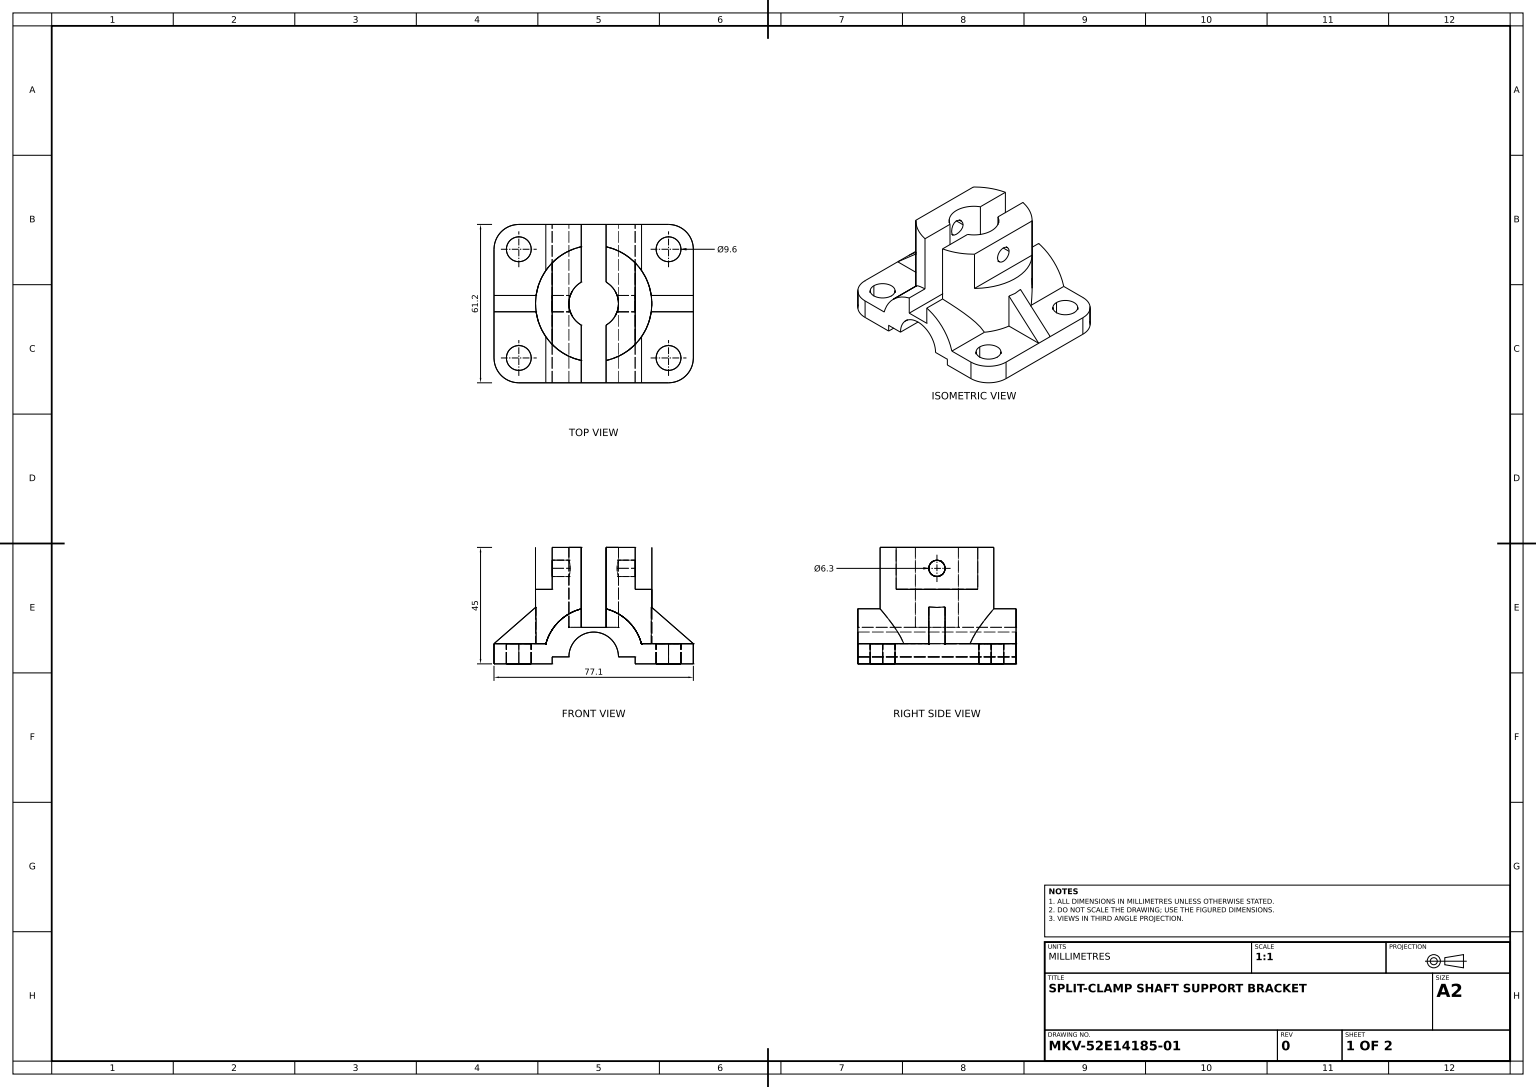
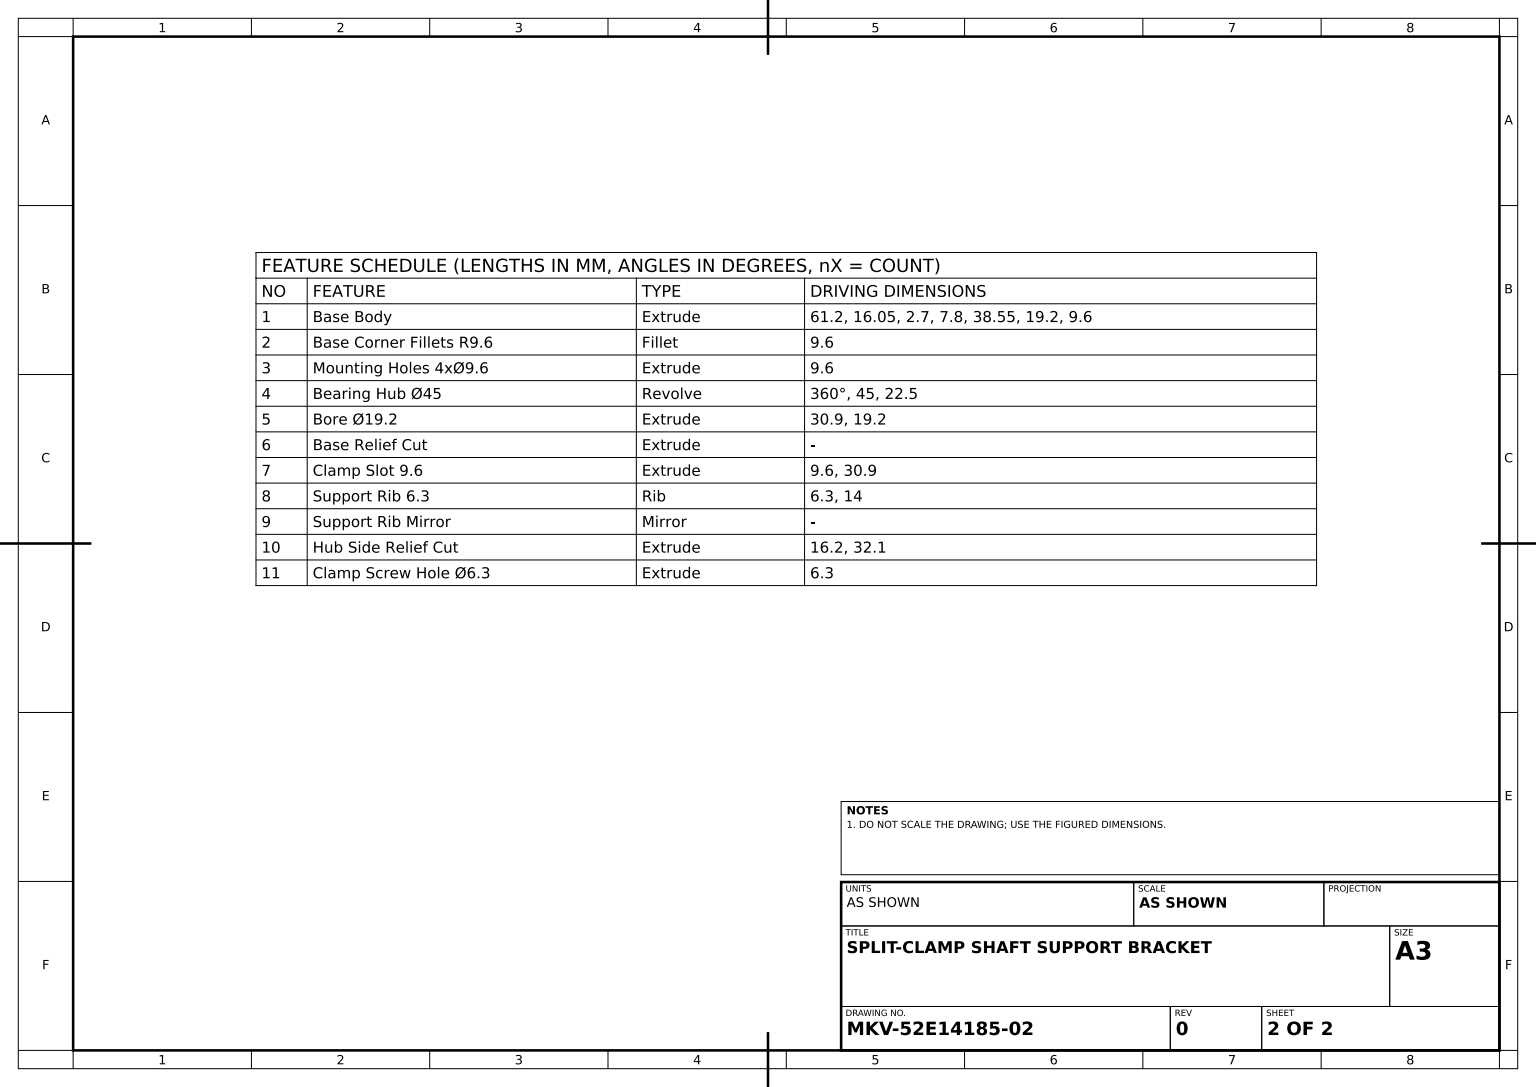
from build123d import *

# Parameters (mm, degrees)
BASE_BODY_DEPTH                 = 30.6
BASE_CORNER_FILLETS_R9_6_R      = 9.6
MOUNTING_HOLES_4X_9_6_REACH     = 53.198
MOUNTING_HOLES_SKETCH_R         = 4.8
BEARING_HUB_PROFILE_SKETCH_W    = 22.5
BEARING_HUB_PROFILE_SKETCH_H    = 37.2
BORE_SKETCH_R                   = 9.6
BORE_19_2_DEPTH                 = 30.9
BASE_RELIEF_CUT_DEPTH           = 84.790408286
CLAMP_SLOT_SKETCH_W             = 9.6
CLAMP_SLOT_SKETCH_H             = 30.9
CLAMP_SLOT_9_6_DEPTH            = 84.790408286
SUPPORT_RIB_6_3_REACH           = 66.898
SUPPORT_RIB_SKETCH_WALL_W       = 153.093978432
SUPPORT_RIB_SKETCH_WALL_H       = 6.3
HUB_SIDE_RELIEF_CUT_DEPTH       = 65.898016261
HUB_SIDE_RELIEF_CUT_DEPTH_BACK  = 65.898016261
HUB_SIDE_RELIEF_SKETCH_W        = 6.45
HUB_SIDE_RELIEF_SKETCH_H        = 16.2
CLAMP_SCREW_HOLE_6_3_DEPTH      = 65.898016261
CLAMP_SCREW_HOLE_6_3_DEPTH_BACK = 65.898016261
CLAMP_SCREW_HOLE_SKETCH_R       = 3.15


with BuildPart() as part:
    # Base Body Profile Sketch → Base Body (new, symmetric)
    with BuildSketch(Plane.XY):
        with BuildLine():
            Line((9.6, 0), (16.05, 0))
            Line((16.05, 0), (16.05, -2.7))
            Line((16.05, -2.7), (38.55, -2.7))
            Line((38.55, -2.7), (38.55, 5.1))
            Line((38.55, 5.1), (18.510267421, 5.1))
            ThreePointArc((18.510267421, 5.1), (0, 19.2), (-18.510267421, 5.1))
            Line((-18.510267421, 5.1), (-38.55, 5.1))
            Line((-38.55, 5.1), (-38.55, -2.7))
            Line((-38.55, -2.7), (-16.05, -2.7))
            Line((-16.05, -2.7), (-16.05, 0))
            Line((-16.05, 0), (-9.6, 0))
            ThreePointArc((-9.6, 0), (0, 9.6), (9.6, 0))
        make_face()
    extrude(amount=BASE_BODY_DEPTH, both=True)

    # Base Corner Fillets R9.6
    base_corner_fillets_r9_6_edges = [part.edges().sort_by_distance(p)[0] for p in [
        (-38.55, 1.2, -30.6),
        (38.55, 1.2, -30.6),
        (38.55, 1.2, 30.6),
        (-38.55, 1.2, 30.6),
    ]]
    fillet(base_corner_fillets_r9_6_edges, radius=BASE_CORNER_FILLETS_R9_6_R)

    # Mounting Holes Sketch → Mounting Holes 4xØ9.6 (cut, up to next)
    with BuildSketch(Plane(origin=(0, 5.1, 0), x_dir=(1, 0, 0), z_dir=(0, 1, 0)), mode=Mode.PRIVATE) as mounting_holes_4x_9_6_sk1:
        with Locations(Location((-28.95, 21, 0), (0, 0, 180))):
            Circle(MOUNTING_HOLES_SKETCH_R)
    mounting_holes_4x_9_6_tool1 = extrude(mounting_holes_4x_9_6_sk1.sketch, amount=-MOUNTING_HOLES_4X_9_6_REACH, mode=Mode.PRIVATE) & part.part
    # Mounting Holes Sketch → Mounting Holes 4xØ9.6 (cut, up to next)
    with BuildSketch(Plane(origin=(0, 5.1, 0), x_dir=(1, 0, 0), z_dir=(0, 1, 0)), mode=Mode.PRIVATE) as mounting_holes_4x_9_6_sk2:
        with Locations(Location((-28.95, -21, 0), (0, 0, 180))):
            Circle(MOUNTING_HOLES_SKETCH_R)
    mounting_holes_4x_9_6_tool2 = extrude(mounting_holes_4x_9_6_sk2.sketch, amount=-MOUNTING_HOLES_4X_9_6_REACH, mode=Mode.PRIVATE) & part.part
    # Mounting Holes Sketch → Mounting Holes 4xØ9.6 (cut, up to next)
    with BuildSketch(Plane(origin=(0, 5.1, 0), x_dir=(1, 0, 0), z_dir=(0, 1, 0)), mode=Mode.PRIVATE) as mounting_holes_4x_9_6_sk3:
        with Locations(Location((28.95, -21, 0), (0, 0, 180))):
            Circle(MOUNTING_HOLES_SKETCH_R)
    mounting_holes_4x_9_6_tool3 = extrude(mounting_holes_4x_9_6_sk3.sketch, amount=-MOUNTING_HOLES_4X_9_6_REACH, mode=Mode.PRIVATE) & part.part
    # Mounting Holes Sketch → Mounting Holes 4xØ9.6 (cut, up to next)
    with BuildSketch(Plane(origin=(0, 5.1, 0), x_dir=(1, 0, 0), z_dir=(0, 1, 0)), mode=Mode.PRIVATE) as mounting_holes_4x_9_6_sk4:
        with Locations(Location((28.95, 21, 0), (0, 0, 180))):
            Circle(MOUNTING_HOLES_SKETCH_R)
    mounting_holes_4x_9_6_tool4 = extrude(mounting_holes_4x_9_6_sk4.sketch, amount=-MOUNTING_HOLES_4X_9_6_REACH, mode=Mode.PRIVATE) & part.part
    add(mounting_holes_4x_9_6_tool1.solids().sort_by_distance((-28.95, 5.1, -21))[0], mode=Mode.SUBTRACT)
    add(mounting_holes_4x_9_6_tool2.solids().sort_by_distance((-28.95, 5.1, 21))[0], mode=Mode.SUBTRACT)
    add(mounting_holes_4x_9_6_tool3.solids().sort_by_distance((28.95, 5.1, 21))[0], mode=Mode.SUBTRACT)
    add(mounting_holes_4x_9_6_tool4.solids().sort_by_distance((28.95, 5.1, -21))[0], mode=Mode.SUBTRACT)

    # Bearing Hub Profile Sketch → Bearing Hub Ø45 (revolve)
    with BuildSketch(Plane.XY, mode=Mode.PRIVATE) as bearing_hub_45_sk:
        with Locations((11.25, 23.7)):
            Rectangle(BEARING_HUB_PROFILE_SKETCH_W, BEARING_HUB_PROFILE_SKETCH_H)
    revolve(bearing_hub_45_sk.sketch.rotate(Axis((0, 5.1, 0), (0, 1, 0)), 90), axis=Axis((0, 5.1, 0), (0, 1, 0)))

    # Bore Sketch → Bore Ø19.2 (cut)
    with BuildSketch(Plane(origin=(0, 42.3, 0), x_dir=(1, 0, 0), z_dir=(0, 1, 0))):
        with Locations(Location((0, 0, 0), (0, 0, 270))):
            Circle(BORE_SKETCH_R)
    extrude(amount=-BORE_19_2_DEPTH, mode=Mode.SUBTRACT)

    # Base Relief Sketch → Base Relief Cut (cut, through all)
    with BuildSketch(Plane.XY.offset(30.6)):
        with BuildLine():
            Line((-9.6, 0), (9.6, 0))
            ThreePointArc((9.6, 0), (0, 9.6), (-9.6, 0))
        make_face()
    extrude(amount=-BASE_RELIEF_CUT_DEPTH, mode=Mode.SUBTRACT)

    # Clamp Slot Sketch → Clamp Slot 9.6 (cut, through all)
    with BuildSketch(Plane.XY.offset(30.6)):
        with Locations((0, 26.85)):
            Rectangle(CLAMP_SLOT_SKETCH_W, CLAMP_SLOT_SKETCH_H)
    extrude(amount=-CLAMP_SLOT_9_6_DEPTH, mode=Mode.SUBTRACT)

    # Support Rib Sketch wall → Support Rib 6.3 (add, up to next)
    with BuildSketch(Plane(origin=(-30.525, 12.1, 0), x_dir=(-0.753593800433, -0.657340386671, 0), z_dir=(0.657340386671, -0.753593800433, 0)), mode=Mode.PRIVATE) as support_rib_6_3_sk1:
        Rectangle(SUPPORT_RIB_SKETCH_WALL_W, SUPPORT_RIB_SKETCH_WALL_H)
    support_rib_6_3_tool1 = extrude(support_rib_6_3_sk1.sketch, amount=SUPPORT_RIB_6_3_REACH, mode=Mode.PRIVATE) - part.part
    support_rib_6_3 = support_rib_6_3_tool1.solids().sort_by_distance((-30.525, 12.1, 0))[0]
    add(support_rib_6_3)

    # Support Rib Mirror: Support Rib 6.3 across plane
    add(support_rib_6_3.mirror(Plane(origin=(0, 0, 0), x_dir=(0, 0, 1), z_dir=(1, 0, 0))))

    # Hub Side Relief Sketch → Hub Side Relief Cut (cut, two sides: drawn at the far end of the back side and taken through both)
    with BuildSketch(Plane.XY.offset(-HUB_SIDE_RELIEF_CUT_DEPTH_BACK)):
        with Locations((-19.275, 34.2)):
            Rectangle(HUB_SIDE_RELIEF_SKETCH_W, HUB_SIDE_RELIEF_SKETCH_H)
        with Locations((19.275, 34.2)):
            Rectangle(HUB_SIDE_RELIEF_SKETCH_W, HUB_SIDE_RELIEF_SKETCH_H)
    extrude(amount=HUB_SIDE_RELIEF_CUT_DEPTH + HUB_SIDE_RELIEF_CUT_DEPTH_BACK, mode=Mode.SUBTRACT)

    # Clamp Screw Hole Sketch → Clamp Screw Hole Ø6.3 (cut, two sides: drawn at the far end of the back side and taken through both)
    with BuildSketch(Plane(origin=(0, 0, 0), x_dir=(0, 0, -1), z_dir=(1, 0, 0)).offset(-CLAMP_SCREW_HOLE_6_3_DEPTH_BACK)):
        with Locations((0, 34.2)):
            Circle(CLAMP_SCREW_HOLE_SKETCH_R)
    extrude(amount=CLAMP_SCREW_HOLE_6_3_DEPTH + CLAMP_SCREW_HOLE_6_3_DEPTH_BACK, mode=Mode.SUBTRACT)


solid = part.part
